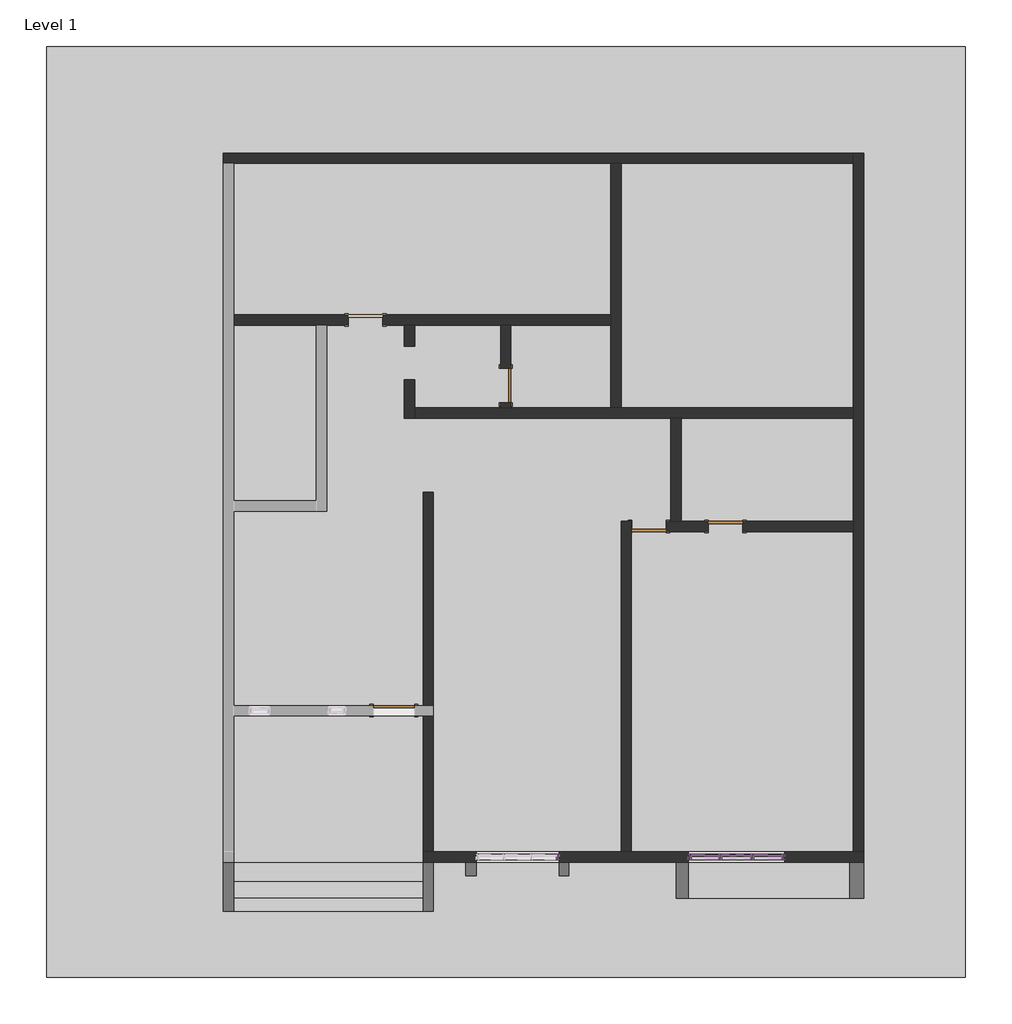
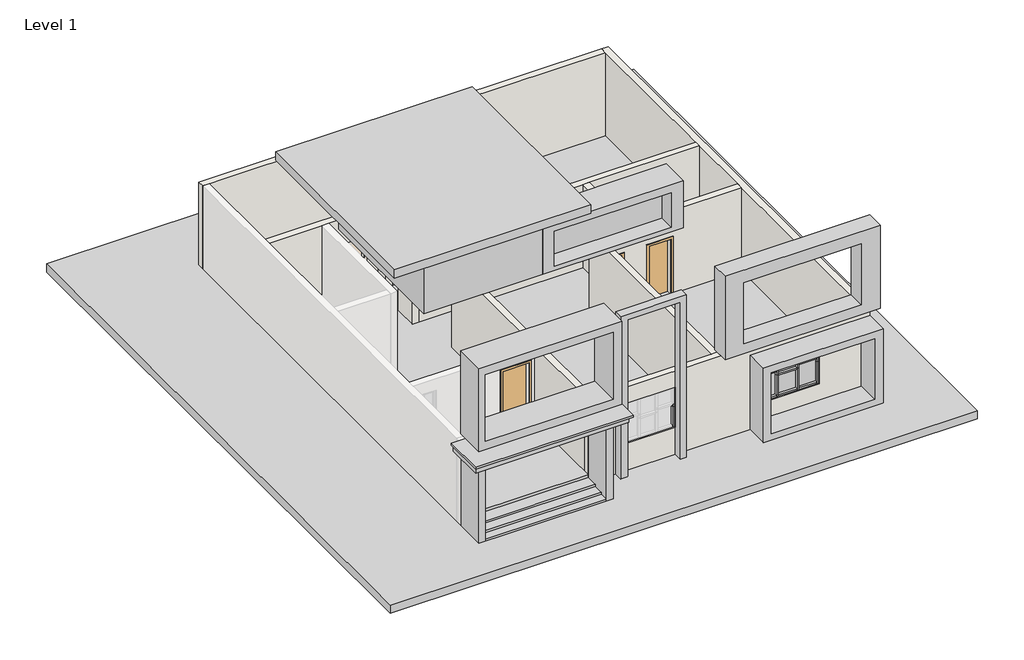
# One storey, part 2 of 2: 23 members, 14 walls, 6 plates, 4 doors, 4 proxies.
"""IFC4 building model written with IfcOpenShell, lengths in millimetres."""

from ifc_helpers import new_model, si_unit, frame, origin, origin_with_axes, place, context, project, spatial, polyline, outline, extrude, faceted_brep, transform, mapped, element, save
from components import generic_models_1_generic_models_1_6e4baba8, generic_models_2_generic_models_2_e7d0f1f0, generic_models_3_generic_models_3_8d7ffd4d, generic_models_4_generic_models_4_0081fb0e, door_a1484949, door_0ca8825f, member_fb13da3b, member_e61db9c9, member_f8dc38bf, member_876f8f00, member_b8383707, member_3f0e0172, member_d4cc7fbf, member_5215b92c, member_f6f0dfdd, member_e53b78c9, member_ccd4d8c6, member_f274020e, system_panel_glazed_23e43b4f, system_panel_glazed_5b2e8898, system_panel_glazed_52878f21, system_panel_glazed_aefe9f20

model = new_model("IFC4")

# Units and contexts
model_context = context("Model", 3, world=origin())
ifc_project = project(units=[si_unit("LENGTHUNIT", "METRE", prefix="MILLI")], contexts=[model_context])

# Site, building, storey
site = spatial("IfcSite", under=ifc_project)
building = spatial("IfcBuilding", under=site)
storey = spatial("IfcBuildingStorey", under=building, Name="Level 1", Elevation=0.0)

# Proxies
placement = place(None, origin())
generic_models_1_generic_models_1_shape = generic_models_1_generic_models_1_6e4baba8(model_context)
element("IfcBuildingElementProxy", 1, Name="Generic Models 1 : Generic Models 1", ObjectType="Generic Models 1 : Generic Models 1", at=placement, inside=storey, context=model_context, shape_type="MappedRepresentation", body=[
    mapped(generic_models_1_generic_models_1_shape, transform((0.0, 0.0, 0.0), x_axis=(1.0, 0.0, 0.0), y_axis=(0.0, 1.0, 0.0), z_axis=(0.0, 0.0, 1.0))),
])
generic_models_2_generic_models_2_shape = generic_models_2_generic_models_2_e7d0f1f0(model_context)
element("IfcBuildingElementProxy", 2, Name="Generic Models 2 : Generic Models 2", ObjectType="Generic Models 2 : Generic Models 2", at=placement, inside=storey, context=model_context, shape_type="MappedRepresentation", body=[
    mapped(generic_models_2_generic_models_2_shape, transform((0.0, 0.0, 0.0), x_axis=(1.0, 0.0, 0.0), y_axis=(0.0, 1.0, 0.0), z_axis=(0.0, 0.0, 1.0))),
])
generic_models_3_generic_models_3_shape = generic_models_3_generic_models_3_8d7ffd4d(model_context)
element("IfcBuildingElementProxy", 3, Name="Generic Models 3 : Generic Models 3", ObjectType="Generic Models 3 : Generic Models 3", at=placement, inside=storey, context=model_context, shape_type="MappedRepresentation", body=[
    mapped(generic_models_3_generic_models_3_shape, transform((0.0, 0.0, 0.0), x_axis=(1.0, 0.0, 0.0), y_axis=(0.0, 1.0, 0.0), z_axis=(0.0, 0.0, 1.0))),
])
generic_models_4_generic_models_4_shape = generic_models_4_generic_models_4_0081fb0e(model_context)
element("IfcBuildingElementProxy", 4, Name="Generic Models 4 : Generic Models 4", ObjectType="Generic Models 4 : Generic Models 4", at=placement, inside=storey, context=model_context, shape_type="MappedRepresentation", body=[
    mapped(generic_models_4_generic_models_4_shape, transform((0.0, 0.0, 0.0), x_axis=(1.0, 0.0, 0.0), y_axis=(0.0, 1.0, 0.0), z_axis=(0.0, 0.0, 1.0))),
])

# Doors
door_shape = door_a1484949(model_context)
element("IfcDoor", 5, ObjectType="Single-Flush : 30\" x 80\"", at=placement, inside=storey, context=model_context, shape_type="MappedRepresentation", body=[
    mapped(door_shape, transform((-9765.7403308, -5925.8518738, 0.0), x_axis=(-1.0, 0.0, 0.0), y_axis=(0.0, -1.0, 0.0), z_axis=(0.0, 0.0, 1.0))),
])
element("IfcDoor", 6, ObjectType="Single-Flush : 30\" x 80\"", at=placement, inside=storey, context=model_context, shape_type="MappedRepresentation", body=[
    mapped(door_shape, transform((-8076.6403308, -5925.8518738, 0.0), x_axis=(1.0, 0.0, 0.0), y_axis=(0.0, 1.0, 0.0), z_axis=(0.0, 0.0, 1.0))),
])
element("IfcDoor", 7, ObjectType="Single-Flush : 30\" x 80\"", at=placement, inside=storey, context=model_context, shape_type="MappedRepresentation", body=[
    mapped(door_shape, transform((-12940.7403308, -2801.6518738, 0.0), x_axis=(0.0, -1.0, 0.0), y_axis=(1.0, 0.0, 0.0), z_axis=(0.0, 0.0, 1.0))),
])
door_2_shape = door_0ca8825f(model_context)
element("IfcDoor", 8, ObjectType="Single-Flush : 36\" x 84\"", at=placement, inside=storey, context=model_context, shape_type="MappedRepresentation", body=[
    mapped(door_2_shape, transform((-15417.2403308, -10002.5518738, 381.0), x_axis=(1.0, 0.0, 0.0), y_axis=(0.0, 1.0, 0.0), z_axis=(0.0, 0.0, 1.0))),
])

# Members
member_shape = member_fb13da3b(model_context)
element("IfcMember", 9, ObjectType="Rectangular Mullion : 2.5\" x 5\" rectangular", at=placement, inside=storey, context=model_context, shape_type="MappedRepresentation", body=[
    mapped(member_shape, transform((-11759.6403308, -13241.0518738, 1723.8543679), x_axis=(1.0, 0.0, 0.0), y_axis=(0.0, -1.0, 0.0), z_axis=(0.0, 0.0, -1.0))),
])
member_2_shape = member_e61db9c9(model_context)
element("IfcMember", 10, ObjectType="Rectangular Mullion : 2.5\" x 5\" rectangular", at=placement, inside=storey, context=model_context, shape_type="MappedRepresentation", body=[
    mapped(member_2_shape, transform((-11759.6403308, -13241.0518738, 987.5576115), x_axis=(1.0, 0.0, 0.0), y_axis=(0.0, -1.0, 0.0), z_axis=(0.0, 0.0, -1.0))),
])
member_3_shape = member_f8dc38bf(model_context)
element("IfcMember", 11, ObjectType="Rectangular Mullion : 2.5\" x 5\" rectangular", at=placement, inside=storey, context=model_context, shape_type="MappedRepresentation", body=[
    mapped(member_3_shape, transform((-6832.0403308, -13241.0518738, 1778.0119563), x_axis=(0.0, 0.0, 1.0), y_axis=(0.0, -1.0, 0.0), z_axis=(1.0, 0.0, 0.0))),
])
element("IfcMember", 12, ObjectType="Rectangular Mullion : 2.5\" x 5\" rectangular", at=placement, inside=storey, context=model_context, shape_type="MappedRepresentation", body=[
    mapped(member_3_shape, transform((-8222.6903308, -13241.0518738, 1778.0119563), x_axis=(0.0, 0.0, 1.0), y_axis=(0.0, -1.0, 0.0), z_axis=(1.0, 0.0, 0.0))),
])
member_4_shape = member_876f8f00(model_context)
element("IfcMember", 13, ObjectType="Rectangular Mullion : 2.5\" x 5\" rectangular", at=placement, inside=storey, context=model_context, shape_type="MappedRepresentation", body=[
    mapped(member_4_shape, transform((-8902.1403308, -13241.0518738, 1778.0119563), x_axis=(-1.0, 0.0, 0.0), y_axis=(0.0, -1.0, 0.0), z_axis=(0.0, 0.0, 1.0))),
])
member_5_shape = member_b8383707(model_context)
element("IfcMember", 14, ObjectType="Rectangular Mullion : 2.5\" x 5\" rectangular", at=placement, inside=storey, context=model_context, shape_type="MappedRepresentation", body=[
    mapped(member_5_shape, transform((-8190.9403308, -13241.0518738, 1778.0119563), x_axis=(1.0, 0.0, 0.0), y_axis=(0.0, -1.0, 0.0), z_axis=(0.0, 0.0, -1.0))),
])
element("IfcMember", 15, ObjectType="Rectangular Mullion : 2.5\" x 5\" rectangular", at=placement, inside=storey, context=model_context, shape_type="MappedRepresentation", body=[
    mapped(member_5_shape, transform((-7479.7403308, -13241.0518738, 1778.0119563), x_axis=(1.0, 0.0, 0.0), y_axis=(0.0, -1.0, 0.0), z_axis=(0.0, 0.0, -1.0))),
])
member_6_shape = member_3f0e0172(model_context)
element("IfcMember", 16, ObjectType="Rectangular Mullion : 2.5\" x 5\" rectangular", at=placement, inside=storey, context=model_context, shape_type="MappedRepresentation", body=[
    mapped(member_6_shape, transform((-8222.6903308, -13241.0518738, 2474.9563458), x_axis=(0.0, 0.0, 1.0), y_axis=(0.0, -1.0, 0.0), z_axis=(1.0, 0.0, 0.0))),
])
element("IfcMember", 17, ObjectType="Rectangular Mullion : 2.5\" x 5\" rectangular", at=placement, inside=storey, context=model_context, shape_type="MappedRepresentation", body=[
    mapped(member_6_shape, transform((-6832.0403308, -13241.0518738, 2474.9563458), x_axis=(0.0, 0.0, 1.0), y_axis=(0.0, -1.0, 0.0), z_axis=(1.0, 0.0, 0.0))),
])
member_7_shape = member_d4cc7fbf(model_context)
element("IfcMember", 18, ObjectType="Rectangular Mullion : 2.5\" x 5\" rectangular", at=placement, inside=storey, context=model_context, shape_type="MappedRepresentation", body=[
    mapped(member_7_shape, transform((-8902.1403308, -13241.0518738, 2474.9563458), x_axis=(-1.0, 0.0, 0.0), y_axis=(0.0, -1.0, 0.0), z_axis=(0.0, 0.0, 1.0))),
])
element("IfcMember", 19, ObjectType="Rectangular Mullion : 2.5\" x 5\" rectangular", at=placement, inside=storey, context=model_context, shape_type="MappedRepresentation", body=[
    mapped(member_4_shape, transform((-6768.5403308, -13241.0518738, 1625.6119563), x_axis=(1.0, 0.0, 0.0), y_axis=(0.0, -1.0, 0.0), z_axis=(0.0, 0.0, -1.0))),
])
element("IfcMember", 20, ObjectType="Rectangular Mullion : 2.5\" x 5\" rectangular", at=placement, inside=storey, context=model_context, shape_type="MappedRepresentation", body=[
    mapped(member_7_shape, transform((-6768.5403308, -13241.0518738, 1778.0119563), x_axis=(1.0, 0.0, 0.0), y_axis=(0.0, -1.0, 0.0), z_axis=(0.0, 0.0, -1.0))),
])
member_8_shape = member_5215b92c(model_context)
element("IfcMember", 21, ObjectType="Rectangular Mullion : 2.5\" x 5\" rectangular", at=placement, inside=storey, context=model_context, shape_type="MappedRepresentation", body=[
    mapped(member_8_shape, transform((-7511.4903308, -13241.0518738, 2474.9563458), x_axis=(0.0, 0.0, 1.0), y_axis=(0.0, -1.0, 0.0), z_axis=(1.0, 0.0, 0.0))),
])
member_9_shape = member_f6f0dfdd(model_context)
element("IfcMember", 22, ObjectType="Rectangular Mullion : 2.5\" x 5\" rectangular", at=placement, inside=storey, context=model_context, shape_type="MappedRepresentation", body=[
    mapped(member_9_shape, transform((-8190.9403308, -13241.0518738, 1625.6119563), x_axis=(1.0, 0.0, 0.0), y_axis=(0.0, -1.0, 0.0), z_axis=(0.0, 0.0, -1.0))),
])
element("IfcMember", 23, ObjectType="Rectangular Mullion : 2.5\" x 5\" rectangular", at=placement, inside=storey, context=model_context, shape_type="MappedRepresentation", body=[
    mapped(member_9_shape, transform((-7479.7403308, -13241.0518738, 1625.6119563), x_axis=(1.0, 0.0, 0.0), y_axis=(0.0, -1.0, 0.0), z_axis=(0.0, 0.0, -1.0))),
])
member_10_shape = member_e53b78c9(model_context)
element("IfcMember", 24, ObjectType="Rectangular Mullion : 2.5\" x 5\" rectangular", at=placement, inside=storey, context=model_context, shape_type="MappedRepresentation", body=[
    mapped(member_10_shape, transform((-7511.4903308, -13241.0518738, 1625.6119563), x_axis=(0.0, 0.0, 1.0), y_axis=(0.0, -1.0, 0.0), z_axis=(1.0, 0.0, 0.0))),
])
member_11_shape = member_ccd4d8c6(model_context)
element("IfcMember", 25, ObjectType="Rectangular Mullion : 2.5\" x 5\" rectangular", at=placement, inside=storey, context=model_context, shape_type="MappedRepresentation", body=[
    mapped(member_11_shape, transform((-8190.9403308, -13241.0518738, 827.0675668), x_axis=(1.0, 0.0, 0.0), y_axis=(0.0, -1.0, 0.0), z_axis=(0.0, 0.0, -1.0))),
])
element("IfcMember", 26, ObjectType="Rectangular Mullion : 2.5\" x 5\" rectangular", at=placement, inside=storey, context=model_context, shape_type="MappedRepresentation", body=[
    mapped(member_11_shape, transform((-7479.7403308, -13241.0518738, 827.0675668), x_axis=(1.0, 0.0, 0.0), y_axis=(0.0, -1.0, 0.0), z_axis=(0.0, 0.0, -1.0))),
])
element("IfcMember", 27, ObjectType="Rectangular Mullion : 2.5\" x 5\" rectangular", at=placement, inside=storey, context=model_context, shape_type="MappedRepresentation", body=[
    mapped(member_6_shape, transform((-7447.9903308, -13241.0518738, 827.0675668), x_axis=(0.0, 0.0, -1.0), y_axis=(0.0, -1.0, 0.0), z_axis=(-1.0, 0.0, 0.0))),
])
element("IfcMember", 28, ObjectType="Rectangular Mullion : 2.5\" x 5\" rectangular", at=placement, inside=storey, context=model_context, shape_type="MappedRepresentation", body=[
    mapped(member_6_shape, transform((-8838.6403308, -13241.0518738, 827.0675668), x_axis=(0.0, 0.0, -1.0), y_axis=(0.0, -1.0, 0.0), z_axis=(-1.0, 0.0, 0.0))),
])
element("IfcMember", 29, ObjectType="Rectangular Mullion : 2.5\" x 5\" rectangular", at=placement, inside=storey, context=model_context, shape_type="MappedRepresentation", body=[
    mapped(member_8_shape, transform((-8159.1903308, -13241.0518738, 827.0675668), x_axis=(0.0, 0.0, -1.0), y_axis=(0.0, -1.0, 0.0), z_axis=(-1.0, 0.0, 0.0))),
])
member_12_shape = member_f274020e(model_context)
element("IfcMember", 30, ObjectType="Rectangular Mullion : 2.5\" x 5\" rectangular", at=placement, inside=storey, context=model_context, shape_type="MappedRepresentation", body=[
    mapped(member_12_shape, transform((-8902.1403308, -13241.0518738, 1625.6119563), x_axis=(-1.0, 0.0, 0.0), y_axis=(0.0, -1.0, 0.0), z_axis=(0.0, 0.0, 1.0))),
])
element("IfcMember", 31, ObjectType="Rectangular Mullion : 2.5\" x 5\" rectangular", at=placement, inside=storey, context=model_context, shape_type="MappedRepresentation", body=[
    mapped(member_12_shape, transform((-6768.5403308, -13241.0518738, 827.0675668), x_axis=(1.0, 0.0, 0.0), y_axis=(0.0, -1.0, 0.0), z_axis=(0.0, 0.0, -1.0))),
])

# Plates
system_panel_glazed_shape = system_panel_glazed_23e43b4f(model_context)
element("IfcPlate", 32, ObjectType="System Panel : Glazed", at=placement, inside=storey, context=model_context, shape_type="MappedRepresentation", body=[
    mapped(system_panel_glazed_shape, transform((-8530.6653308, -13241.0518738, 1809.7619563), x_axis=(1.0, 0.0, 0.0), y_axis=(0.0, 1.0, 0.0), z_axis=(0.0, 0.0, 1.0))),
])
element("IfcPlate", 33, ObjectType="System Panel : Glazed", at=placement, inside=storey, context=model_context, shape_type="MappedRepresentation", body=[
    mapped(system_panel_glazed_shape, transform((-7140.0153308, -13241.0518738, 1809.7619563), x_axis=(1.0, 0.0, 0.0), y_axis=(0.0, 1.0, 0.0), z_axis=(0.0, 0.0, 1.0))),
])
system_panel_glazed_2_shape = system_panel_glazed_5b2e8898(model_context)
element("IfcPlate", 34, ObjectType="System Panel : Glazed", at=placement, inside=storey, context=model_context, shape_type="MappedRepresentation", body=[
    mapped(system_panel_glazed_2_shape, transform((-7835.3403308, -13241.0518738, 1657.3619563), x_axis=(1.0, 0.0, 0.0), y_axis=(0.0, 1.0, 0.0), z_axis=(0.0, 0.0, 1.0))),
])
system_panel_glazed_3_shape = system_panel_glazed_52878f21(model_context)
element("IfcPlate", 35, ObjectType="System Panel : Glazed", at=placement, inside=storey, context=model_context, shape_type="MappedRepresentation", body=[
    mapped(system_panel_glazed_3_shape, transform((-8530.6653308, -13241.0518738, 890.5675668), x_axis=(1.0, 0.0, 0.0), y_axis=(0.0, 1.0, 0.0), z_axis=(0.0, 0.0, 1.0))),
])
element("IfcPlate", 36, ObjectType="System Panel : Glazed", at=placement, inside=storey, context=model_context, shape_type="MappedRepresentation", body=[
    mapped(system_panel_glazed_3_shape, transform((-7140.0153308, -13241.0518738, 890.5675668), x_axis=(1.0, 0.0, 0.0), y_axis=(0.0, 1.0, 0.0), z_axis=(0.0, 0.0, 1.0))),
])
system_panel_glazed_4_shape = system_panel_glazed_aefe9f20(model_context)
element("IfcPlate", 37, ObjectType="System Panel : Glazed", at=placement, inside=storey, context=model_context, shape_type="MappedRepresentation", body=[
    mapped(system_panel_glazed_4_shape, transform((-7835.3403308, -13241.0518738, 890.5675668), x_axis=(1.0, 0.0, 0.0), y_axis=(0.0, 1.0, 0.0), z_axis=(0.0, 0.0, 1.0))),
])

# Walls
element("IfcWall", 38, ObjectType="9\"", at=placement, inside=storey, context=model_context, shape_type="Brep", body=[
    faceted_brep([(-5015.9403308, -13126.7518738, 0.0), (-5015.9403308, 2341.8481262, 0.0), (-5015.9403308, 2341.8481262, 3048.0), (-5015.9403308, -13126.7518738, 3048.0), (-5244.5403308, -13126.7518738, 0.0), (-5244.5403308, -13126.7518738, 3048.0), (-5244.5403308, -6040.1518738, 3048.0), (-5244.5403308, -5811.5518738, 3048.0), (-5244.5403308, -3525.5518738, 3048.0), (-5244.5403308, -3296.9518738, 3048.0), (-5244.5403308, 2113.2481262, 3048.0), (-5244.5403308, 2341.8481262, 3048.0), (-5244.5403308, 2341.8481262, 0.0), (-5244.5403308, 2113.2481262, 0.0), (-5244.5403308, -3296.9518738, 0.0), (-5244.5403308, -3525.5518738, 0.0), (-5244.5403308, -5811.5518738, 0.0), (-5244.5403308, -6040.1518738, 0.0)], [[[0, 1, 2, 3]], [[4, 5, 6, 7, 8, 9, 10, 11, 12, 13, 14, 15, 16, 17]], [[1, 0, 4, 17, 16, 15, 14, 13, 12]], [[3, 2, 11, 10, 9, 8, 7, 6, 5]], [[0, 3, 5, 4]], [[2, 1, 12, 11]]]),
])
element("IfcWall", 39, ObjectType="9\"", at=placement, inside=storey, context=model_context, shape_type="Brep", body=[
    faceted_brep([(-5244.5403308, 2341.8481262, 0.0), (-19189.1403308, 2341.8481262, 0.0), (-19189.1403308, 2341.8481262, 3048.0), (-5244.5403308, 2341.8481262, 3048.0), (-5244.5403308, 2113.2481262, 0.0), (-5244.5403308, 2113.2481262, 3048.0), (-10388.0403308, 2113.2481262, 3048.0), (-10616.6403308, 2113.2481262, 3048.0), (-18960.5403308, 2113.2481262, 3048.0), (-19189.1403308, 2113.2481262, 3048.0), (-19189.1403308, 2113.2481262, 0.0), (-18960.5403308, 2113.2481262, 0.0), (-10616.6403308, 2113.2481262, 0.0), (-10388.0403308, 2113.2481262, 0.0)], [[[0, 1, 2, 3]], [[4, 5, 6, 7, 8, 9, 10, 11, 12, 13]], [[1, 0, 4, 13, 12, 11, 10]], [[3, 2, 9, 8, 7, 6, 5]], [[0, 3, 5, 4]], [[2, 1, 10, 9]]]),
])
element("IfcWall", 40, ObjectType="9\"", at=placement, inside=storey, context=model_context, shape_type="SweptSolid", body=[
    extrude(outline(polyline([(-14769.5403308, -13126.7518738), (-14769.5403308, -10116.8518738), (-14540.9403308, -10116.8518738), (-14540.9403308, -13126.7518738), (-14769.5403308, -13126.7518738)])), origin_with_axes(), (0.0, 0.0, 1.0), 3048.0),
])
element("IfcWall", 41, ObjectType="9\"", at=placement, inside=storey, context=model_context, shape_type="SweptSolid", body=[
    extrude(outline(polyline([(-14540.9403308, -5163.8518738), (-14540.9403308, -9888.2518738), (-14769.5403308, -9888.2518738), (-14769.5403308, -5163.8518738), (-14540.9403308, -5163.8518738)])), origin_with_axes(), (0.0, 0.0, 1.0), 3048.0),
])
element("IfcWall", 42, ObjectType="9\"", at=placement, inside=storey, context=model_context, shape_type="Brep", body=[
    faceted_brep([(-10159.4403308, -13126.7518738, 0.0), (-10159.4403308, -6040.1518738, 0.0), (-10159.4403308, -5811.5518738, 0.0), (-10159.4403308, -5811.5518738, 3048.0), (-10159.4403308, -6040.1518738, 3048.0), (-10159.4403308, -13126.7518738, 3048.0), (-10388.0403308, -13126.7518738, 0.0), (-10388.0403308, -13126.7518738, 3048.0), (-10388.0403308, -5811.5518738, 3048.0), (-10388.0403308, -5811.5518738, 0.0)], [[[0, 1, 2, 3, 4, 5]], [[6, 7, 8, 9]], [[2, 1, 0, 6, 9]], [[5, 4, 3, 8, 7]], [[0, 5, 7, 6]], [[3, 2, 9, 8]]]),
])
element("IfcWall", 43, ObjectType="9\"", at=placement, inside=storey, context=model_context, shape_type="Brep", body=[
    faceted_brep([(-7695.6403308, -6040.1518738, 2032.0), (-7695.6403308, -6040.1518738, 0.0), (-5244.5403308, -6040.1518738, 0.0), (-5244.5403308, -6040.1518738, 3048.0), (-10159.4403308, -6040.1518738, 3048.0), (-10159.4403308, -6040.1518738, 0.0), (-10146.7403308, -6040.1518738, 0.0), (-10146.7403308, -6040.1518738, 2032.0), (-9384.7403308, -6040.1518738, 2032.0), (-9384.7403308, -6040.1518738, 0.0), (-8457.6403308, -6040.1518738, 0.0), (-8457.6403308, -6040.1518738, 2032.0), (-5244.5403308, -5811.5518738, 0.0), (-7695.6403308, -5811.5518738, 0.0), (-7695.6403308, -5811.5518738, 2032.0), (-8457.6403308, -5811.5518738, 2032.0), (-8457.6403308, -5811.5518738, 0.0), (-9054.5403308, -5811.5518738, 0.0), (-9283.1403308, -5811.5518738, 0.0), (-9384.7403308, -5811.5518738, 0.0), (-9384.7403308, -5811.5518738, 2032.0), (-10146.7403308, -5811.5518738, 2032.0), (-10146.7403308, -5811.5518738, 0.0), (-10159.4403308, -5811.5518738, 0.0), (-10159.4403308, -5811.5518738, 3048.0), (-9283.1403308, -5811.5518738, 3048.0), (-9054.5403308, -5811.5518738, 3048.0), (-5244.5403308, -5811.5518738, 3048.0)], [[[0, 1, 2, 3, 4, 5, 6, 7, 8, 9, 10, 11]], [[12, 13, 14, 15, 16, 17, 18, 19, 20, 21, 22, 23, 24, 25, 26, 27]], [[23, 22, 6, 5]], [[10, 9, 19, 18, 17, 16]], [[2, 1, 13, 12]], [[4, 3, 27, 26, 25, 24]], [[5, 4, 24, 23]], [[3, 2, 12, 27]], [[7, 6, 22, 21]], [[8, 7, 21, 20]], [[9, 8, 20, 19]], [[14, 13, 1, 0]], [[15, 14, 0, 11]], [[16, 15, 11, 10]]]),
])
element("IfcWall", 44, ObjectType="9\"", at=placement, inside=storey, context=model_context, shape_type="Brep", body=[
    faceted_brep([(-10616.6403308, 2113.2481262, 0.0), (-10616.6403308, -1239.5518738, 0.0), (-10616.6403308, -1468.1518738, 0.0), (-10616.6403308, -3296.9518738, 0.0), (-10616.6403308, -3296.9518738, 3048.0), (-10616.6403308, -1468.1518738, 3048.0), (-10616.6403308, -1239.5518738, 3048.0), (-10616.6403308, 2113.2481262, 3048.0), (-10388.0403308, 2113.2481262, 0.0), (-10388.0403308, 2113.2481262, 3048.0), (-10388.0403308, -3296.9518738, 3048.0), (-10388.0403308, -3296.9518738, 0.0)], [[[0, 1, 2, 3, 4, 5, 6, 7]], [[8, 9, 10, 11]], [[3, 2, 1, 0, 8, 11]], [[7, 6, 5, 4, 10, 9]], [[0, 7, 9, 8]], [[4, 3, 11, 10]]]),
])
element("IfcWall", 45, ObjectType="9\"", at=placement, inside=storey, context=model_context, shape_type="Brep", body=[
    faceted_brep([(-10616.6403308, -1239.5518738, 0.0), (-15664.8903308, -1239.5518738, 0.0), (-15664.8903308, -1239.5518738, 2032.0), (-16426.8903308, -1239.5518738, 2032.0), (-16426.8903308, -1239.5518738, 0.0), (-18960.5403308, -1239.5518738, 0.0), (-18960.5403308, -1239.5518738, 3048.0), (-10616.6403308, -1239.5518738, 3048.0), (-15664.8903308, -1468.1518738, 2032.0), (-15664.8903308, -1468.1518738, 0.0), (-15188.6403308, -1468.1518738, 0.0), (-14960.0403308, -1468.1518738, 0.0), (-13055.0403308, -1468.1518738, 0.0), (-12826.4403308, -1468.1518738, 0.0), (-10616.6403308, -1468.1518738, 0.0), (-10616.6403308, -1468.1518738, 3048.0), (-12826.4403308, -1468.1518738, 3048.0), (-13055.0403308, -1468.1518738, 3048.0), (-14960.0403308, -1468.1518738, 3048.0), (-15188.6403308, -1468.1518738, 3048.0), (-16903.1403308, -1468.1518738, 3048.0), (-17131.7403308, -1468.1518738, 3048.0), (-18960.5403308, -1468.1518738, 3048.0), (-18960.5403308, -1468.1518738, 0.0), (-17131.7403308, -1468.1518738, 0.0), (-16903.1403308, -1468.1518738, 0.0), (-16426.8903308, -1468.1518738, 0.0), (-16426.8903308, -1468.1518738, 2032.0)], [[[0, 1, 2, 3, 4, 5, 6, 7]], [[8, 9, 10, 11, 12, 13, 14, 15, 16, 17, 18, 19, 20, 21, 22, 23, 24, 25, 26, 27]], [[26, 25, 24, 23, 5, 4]], [[14, 13, 12, 11, 10, 9, 1, 0]], [[7, 6, 22, 21, 20, 19, 18, 17, 16, 15]], [[0, 7, 15, 14]], [[6, 5, 23, 22]], [[2, 1, 9, 8]], [[3, 2, 8, 27]], [[4, 3, 27, 26]]]),
])
element("IfcWall", 46, ObjectType="9\"", at=placement, inside=storey, context=model_context, shape_type="SweptSolid", body=[
    extrude(outline(polyline([(-15188.6403308, -1938.0518738), (-15188.6403308, -1468.1518738), (-14960.0403308, -1468.1518738), (-14960.0403308, -1938.0518738), (-15188.6403308, -1938.0518738)])), origin_with_axes(), (0.0, 0.0, 1.0), 3048.0),
])
element("IfcWall", 47, ObjectType="9\"", at=placement, inside=storey, context=model_context, shape_type="Brep", body=[
    faceted_brep([(-14960.0403308, -3525.5518738, 0.0), (-9283.1403308, -3525.5518738, 0.0), (-9054.5403308, -3525.5518738, 0.0), (-5244.5403308, -3525.5518738, 0.0), (-5244.5403308, -3525.5518738, 3048.0), (-9054.5403308, -3525.5518738, 3048.0), (-9283.1403308, -3525.5518738, 3048.0), (-14960.0403308, -3525.5518738, 3048.0), (-14960.0403308, -3296.9518738, 0.0), (-14960.0403308, -3296.9518738, 3048.0), (-13055.0403308, -3296.9518738, 3048.0), (-12826.4403308, -3296.9518738, 3048.0), (-10616.6403308, -3296.9518738, 3048.0), (-10388.0403308, -3296.9518738, 3048.0), (-5244.5403308, -3296.9518738, 3048.0), (-5244.5403308, -3296.9518738, 0.0), (-10388.0403308, -3296.9518738, 0.0), (-10616.6403308, -3296.9518738, 0.0), (-12826.4403308, -3296.9518738, 0.0), (-13055.0403308, -3296.9518738, 0.0)], [[[0, 1, 2, 3, 4, 5, 6, 7]], [[8, 9, 10, 11, 12, 13, 14, 15, 16, 17, 18, 19]], [[3, 2, 1, 0, 8, 19, 18, 17, 16, 15]], [[7, 6, 5, 4, 14, 13, 12, 11, 10, 9]], [[0, 7, 9, 8]], [[4, 3, 15, 14]]]),
])
element("IfcWall", 48, ObjectType="9\"", at=placement, inside=storey, context=model_context, shape_type="SweptSolid", body=[
    extrude(outline(polyline([(-9283.1403308, -5811.5518738), (-9283.1403308, -3525.5518738), (-9054.5403308, -3525.5518738), (-9054.5403308, -5811.5518738), (-9283.1403308, -5811.5518738)])), origin_with_axes(), (0.0, 0.0, 1.0), 3048.0),
])
element("IfcWall", 49, ObjectType="9\"", at=placement, inside=storey, context=model_context, shape_type="SweptSolid", body=[
    extrude(outline(polyline([(-3182.6518738, 2032.0), (-3182.6518738, 0.0), (-3296.9518738, 0.0), (-3296.9518738, 3048.0), (-1468.1518738, 3048.0), (-1468.1518738, 0.0), (-2420.6518738, 0.0), (-2420.6518738, 2032.0), (-3182.6518738, 2032.0)])), frame((-13055.0403308, 0.0, 0.0), z_axis=(1.0, 0.0, 0.0), x_axis=(0.0, 1.0, 0.0)), (0.0, 0.0, 1.0), 228.6),
])
element("IfcWall", 50, ObjectType="9\"", at=placement, inside=storey, context=model_context, shape_type="Brep", body=[
    faceted_brep([(-15188.6403308, -2674.6518738, 0.0), (-15188.6403308, -3525.5518738, 0.0), (-15188.6403308, -3525.5518738, 3048.0), (-15188.6403308, -2674.6518738, 3048.0), (-14960.0403308, -2674.6518738, 0.0), (-14960.0403308, -2674.6518738, 3048.0), (-14960.0403308, -3296.9518738, 3048.0), (-14960.0403308, -3525.5518738, 3048.0), (-14960.0403308, -3525.5518738, 0.0), (-14960.0403308, -3296.9518738, 0.0)], [[[0, 1, 2, 3]], [[4, 5, 6, 7, 8, 9]], [[1, 0, 4, 9, 8]], [[3, 2, 7, 6, 5]], [[0, 3, 5, 4]], [[2, 1, 8, 7]]]),
])
element("IfcWall", 51, ObjectType="9\"", at=placement, inside=storey, context=model_context, shape_type="Brep", body=[
    faceted_brep([(-14769.5403308, -13355.3518738, 0.0), (-5015.9403308, -13355.3518738, 0.0), (-5015.9403308, -13355.3518738, 3048.0), (-14769.5403308, -13355.3518738, 3048.0), (-13588.4403308, -13355.3518738, 987.5576115), (-13588.4403308, -13355.3518738, 2460.1511243), (-11759.6403308, -13355.3518738, 2460.1511243), (-11759.6403308, -13355.3518738, 987.5576115), (-8902.1403308, -13355.3518738, 827.0675668), (-8902.1403308, -13355.3518738, 2474.9563458), (-6768.5403308, -13355.3518738, 2474.9563458), (-6768.5403308, -13355.3518738, 827.0675668), (-5015.9403308, -13126.7518738, 0.0), (-5244.5403308, -13126.7518738, 0.0), (-10159.4403308, -13126.7518738, 0.0), (-10388.0403308, -13126.7518738, 0.0), (-14540.9403308, -13126.7518738, 0.0), (-14769.5403308, -13126.7518738, 0.0), (-14769.5403308, -13126.7518738, 3048.0), (-14540.9403308, -13126.7518738, 3048.0), (-10388.0403308, -13126.7518738, 3048.0), (-10159.4403308, -13126.7518738, 3048.0), (-5244.5403308, -13126.7518738, 3048.0), (-5015.9403308, -13126.7518738, 3048.0), (-13588.4403308, -13126.7518738, 2460.1511243), (-13588.4403308, -13126.7518738, 987.5576115), (-11759.6403308, -13126.7518738, 987.5576115), (-11759.6403308, -13126.7518738, 2460.1511243), (-8902.1403308, -13126.7518738, 2474.9563458), (-8902.1403308, -13126.7518738, 827.0675668), (-6768.5403308, -13126.7518738, 827.0675668), (-6768.5403308, -13126.7518738, 2474.9563458)], [[[0, 1, 2, 3], [4, 5, 6, 7], [8, 9, 10, 11]], [[12, 13, 14, 15, 16, 17, 18, 19, 20, 21, 22, 23], [24, 25, 26, 27], [28, 29, 30, 31]], [[1, 0, 17, 16, 15, 14, 13, 12]], [[3, 2, 23, 22, 21, 20, 19, 18]], [[0, 3, 18, 17]], [[2, 1, 12, 23]], [[24, 5, 4, 25]], [[5, 24, 27, 6]], [[6, 27, 26, 7]], [[25, 4, 7, 26]], [[8, 29, 28, 9]], [[9, 28, 31, 10]], [[10, 31, 30, 11]], [[29, 8, 11, 30]]]),
])

save(model, "model.ifc")

# Revit data of these elements
# Type "Single-Flush : 30\" x 80\""
#   Type Mark = "5"
#   Construction Type Id = "MDOOR"
#   Assembly Code = "C1020"
#   Analytic Construction = "Metal"
#   Thickness = 0' - 2"
#   Heat Transfer Coefficient (U) = 0.651978 BTU/(h·ft²·°F)
#   Height = 6' - 8"
#   Trim Projection Ext = 0' - 1"
#   Trim Projection Int = 0' - 1"
#   Trim Width = 0' - 3"
#   Width = 2' - 6"
#   Define Thermal Properties by = 1
#   Define Thermal Properties by = 1
#   Door Material = Door - Panel
#   Frame Material = Door - Frame
#   Visual Light Transmittance = 0
#   Solar Heat Gain Coefficient = 0
#   Function = (empty or 0)
#   Wall Closure = (empty or 0)
# Type "Single-Flush : 36\" x 84\""
#   Type Mark = "1"
#   Construction Type Id = "MDOOR"
#   Assembly Code = "C1020"
#   Analytic Construction = "Metal"
#   Thickness = 0' - 2"
#   Heat Transfer Coefficient (U) = 0.651978 BTU/(h·ft²·°F)
#   Height = 7' - 0"
#   Trim Projection Ext = 0' - 1"
#   Trim Projection Int = 0' - 1"
#   Trim Width = 0' - 3"
#   Width = 3' - 0"
#   Define Thermal Properties by = 1
#   Define Thermal Properties by = 1
#   Door Material = Door - Panel
#   Frame Material = Door - Frame
#   Visual Light Transmittance = 0
#   Solar Heat Gain Coefficient = 0
#   Function = (empty or 0)
#   Wall Closure = (empty or 0)
# Type "Rectangular Mullion : 2.5\" x 5\" rectangular"
#   built-in parameter 1007304 = 0.416667 (stored number, unit not read)
#   built-in parameter 1007301 = 0.104167 (stored number, unit not read)
#   built-in parameter 1007300 = 0.104167 (stored number, unit not read)
# Type "System Panel : Glazed"
#   Construction Type Id = "GSP4R"
#   Analytic Construction = "1/8 in Pilkington single glazing"
#   Visual Light Transmittance = 0.9
#   Solar Heat Gain Coefficient = 0.86
#   Heat Transfer Coefficient (U) = 1.18115 BTU/(h·ft²·°F)
#   Define Thermal Properties by = 1
# Type "9\""
#   Assembly Code = "B2010"
#   Layers, outside or top first: 0' - 9" no material (function 1)
# Element 1 (IfcBuildingElementProxy, "Generic Models 1 : Generic Models 1")
#   Phase Created = New Construction
# Element 2 (IfcBuildingElementProxy, "Generic Models 2 : Generic Models 2")
#   Phase Created = New Construction
# Element 3 (IfcBuildingElementProxy, "Generic Models 3 : Generic Models 3")
#   Phase Created = New Construction
# Element 4 (IfcBuildingElementProxy, "Generic Models 4 : Generic Models 4")
#   Phase Created = New Construction
# Elements 5, 6, 7 (IfcDoor, "Single-Flush : 30\" x 80\"")
#   Phase Created = New Construction
#   Materials on its faces: "Door - Frame", "Door - Panel"
# Element 8 (IfcDoor, "Single-Flush : 36\" x 84\"")
#   Phase Created = New Construction
#   Materials on its faces: "Door - Frame", "Door - Panel"
# Elements 9, 10, 11, 12, 13, 14, 15, 16, 17, 18, 19, 20, 21, 22, 23, 24, 25, 26, 27, 28, 29, 30, 31 (IfcMember, "Rectangular Mullion : 2.5\" x 5\" rectangular")
#   Phase Created = New Construction
#   Materials on its faces: "Aluminum"
# Elements 32, 33, 34, 35, 36, 37 (IfcPlate, "System Panel : Glazed")
#   Phase Created = New Construction
#   Materials on its faces: "Glass"
# Elements 38, 39, 40, 41, 42, 43, 44, 45, 46, 47, 48, 49, 50, 51 (IfcWall, "9\"")
#   Top Offset = 0' - 0"
#   Base Offset = 0' - 0"
#   Unconnected Height = 10' - 0"
#   wall height = 10' - 0"
#   Phase Created = New Construction
#   Base Constraint = Level 1
#   Materials on its faces: "Default Wall"
# Materials
#   "Door - Panel": class "Wood", colour RGB 210 159 95, transparency 0, Cost = 0
#   "Door - Frame": colour RGB 118 70 51, transparency 0, Cost = 0
#   "Aluminum": class "Metal", colour RGB 247 247 247, transparency 0, Description = "Aluminum 6061", Cost = 0
#   "Glass": class "Glass", colour RGB 0 128 192, transparency 0.75, Description = "Soda Lime Glass", Cost = 0
#   "Default Wall": colour RGB 128 128 128, transparency 0, Cost = 0
